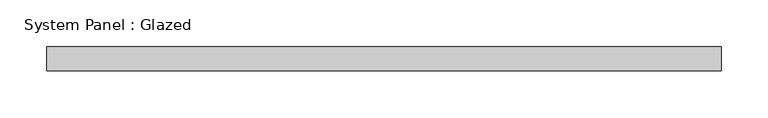
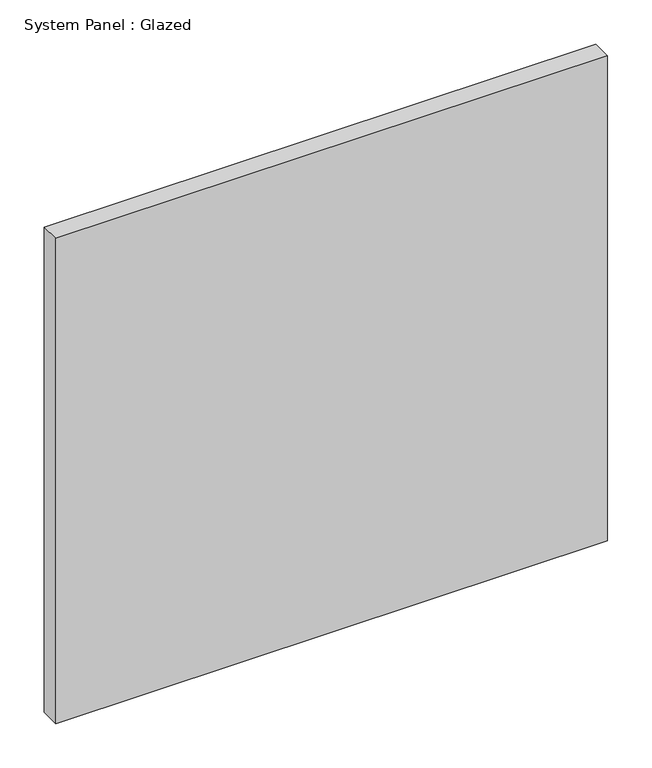
"""IFC4 building model written with IfcOpenShell, lengths in millimetres: plate geometry, System Panel : Glazed."""

from ifc_helpers import new_model, si_unit, origin, origin_with_axes, place, context, project, spatial, polyline, outline, extrude, source, transform, mapped, element, save


def system_panel_glazed_ae16f783(model_context):
    return source(origin(), model_context, "Body", "SweptSolid", [
        extrude(outline(polyline([(358.783438, 19.05), (-358.783438, 19.05), (-358.783438, 44.45), (358.783438, 44.45), (358.783438, 19.05)])), origin_with_axes(), (0.0, 0.0, 1.0), 666.75),
    ])


if __name__ == "__main__":
    model = new_model("IFC4")
    model_context = context("Model", 3, world=origin())
    ifc_project = project(units=[si_unit("LENGTHUNIT", "METRE", prefix="MILLI")], contexts=[model_context])
    site = spatial("IfcSite", under=ifc_project)
    building = spatial("IfcBuilding", under=site)
    placement = place(None, origin())
    system_panel_glazed_shape = system_panel_glazed_ae16f783(model_context)
    element("IfcPlate", 1, ObjectType="System Panel : Glazed", at=placement, inside=building, context=model_context, shape_type="MappedRepresentation", body=[
        mapped(system_panel_glazed_shape, transform((0.0, 0.0, 0.0), x_axis=(1.0, 0.0, 0.0), y_axis=(0.0, 1.0, 0.0), z_axis=(0.0, 0.0, 1.0))),
    ])
    save(model, "model.ifc")

# Revit data of these elements
# Type "System Panel : Glazed"
#   Construction Type Id = "GSP4R"
#   Analytic Construction = "1/8 in Pilkington single glazing"
#   Visual Light Transmittance = 0.9
#   Solar Heat Gain Coefficient = 0.86
#   Heat Transfer Coefficient (U) = 1.18115 BTU/(h·ft²·°F)
# Element 1 (IfcPlate, "System Panel : Glazed")
#   Materials on its faces: "Glass"
# Materials
#   "Glass": class "Glass", colour RGB 0 128 192, transparency 0.75, Description = "Soda Lime Glass", Cost = 0
